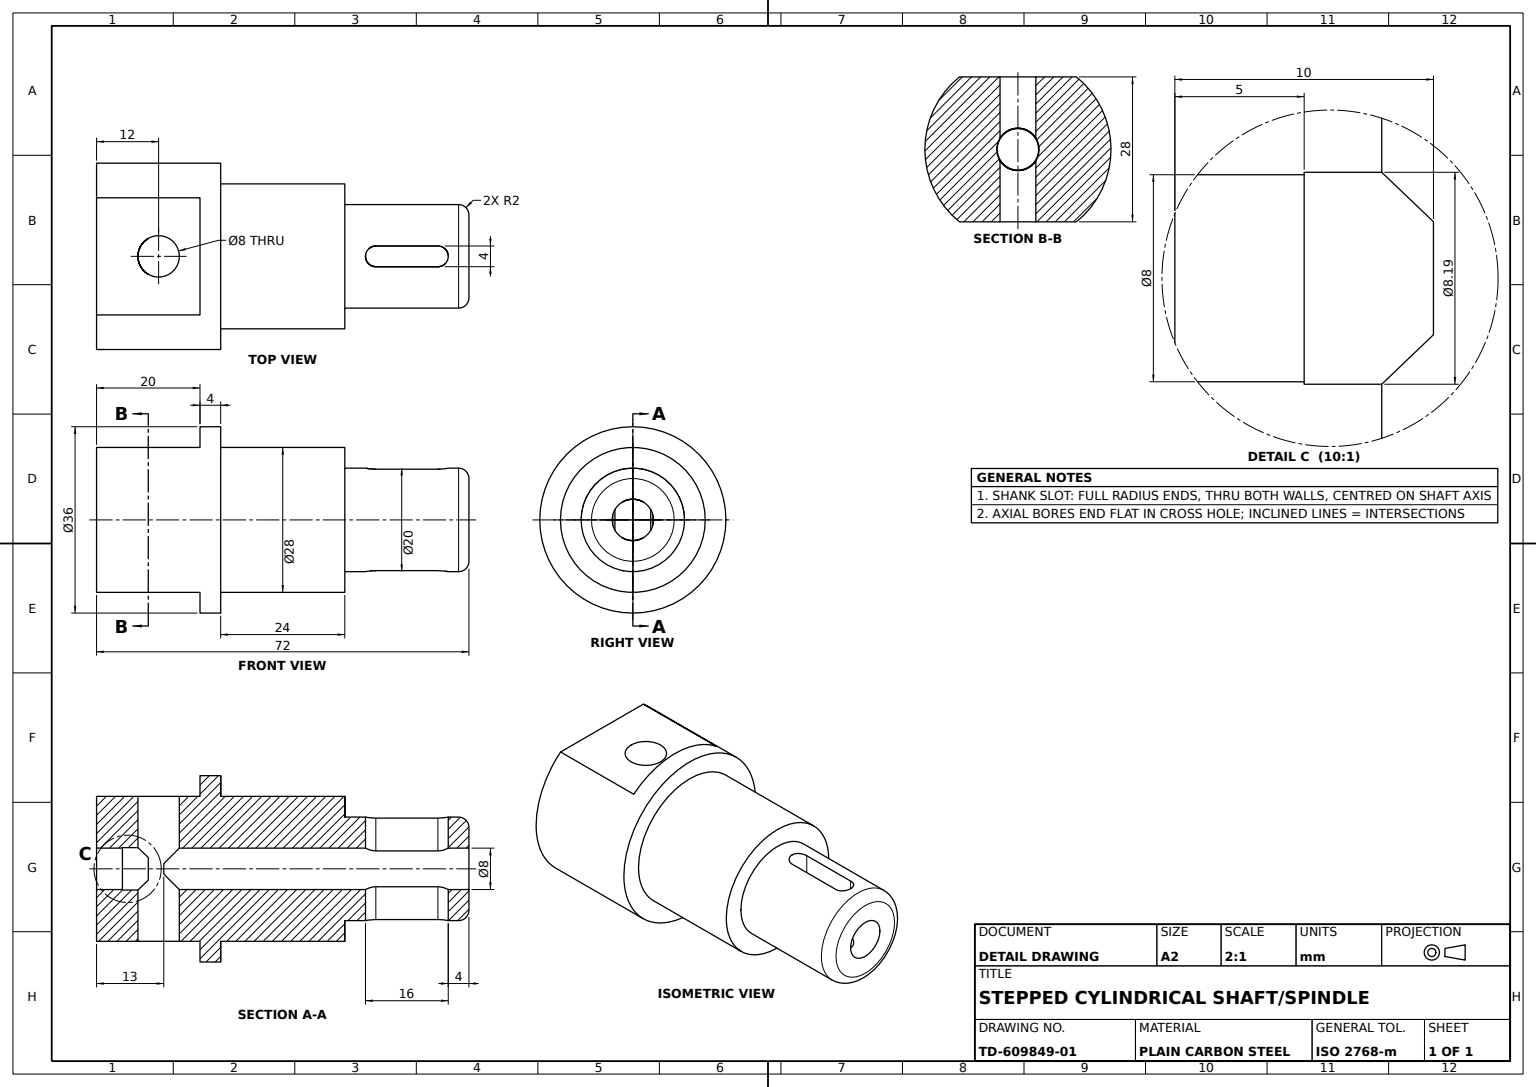
SolidWorks part; units mm, degrees
material "Plain Carbon Steel"
ref_plane "Front Plane" through (0, 0, 0) normal (0, 0, 1) x (1, 0, 0)
ref_plane "Top Plane" through (0, 0, 0) normal (0, 1, 0) x (1, 0, 0)
ref_plane "Right Plane" through (0, 0, 0) normal (1, 0, 0) x (0, 0, -1)
sketch "Shank Ø20 Sketch" plane through (0, 0, 0) normal (0, 1, 0) x (1, 0, 0)
  circle A0 centre (0, 0) radius 10
  dimension "D1" = 20
extrude "Shank Ø20 Step 1" add sketch "Shank Ø20 Sketch" along normal blind 8
sketch "Shank Step 2 Sketch" plane through (0, 8, 0) normal (0, 1, 0) x (1, 0, 0)
  circle A0 centre (0, 0) radius 10
  dimension "D1" = 20
extrude "Shank Ø20 Step 2" add sketch "Shank Step 2 Sketch" along normal blind 8
sketch "Shank Step 3 Sketch" plane through (0, 16, 0) normal (0, 1, 0) x (1, 0, 0)
  circle A0 centre (0, 0) radius 10
  dimension "D1" = 20
extrude "Shank Ø20 Step 3" add sketch "Shank Step 3 Sketch" along normal blind 8
fillet "Shank End Fillet R2" radius 2 1 edges at (0, 24, 10)
sketch "Shank Bore Ø8 Sketch" plane through (0, 24, 0) normal (0, 1, 0) x (1, 0, 0)
  circle A0 centre (0, 0) radius 4
  dimension "D1" = 8
extrude "Shank Bore Ø8 Cut 1" cut sketch "Shank Bore Ø8 Sketch" against normal blind 8
sketch "Shank Bore Cut 2 Sketch" plane through (0, 16, 0) normal (0, 1, 0) x (1, 0, 0)
  circle A0 centre (0, 0) radius 4
  dimension "D1" = 8
extrude "Shank Bore Ø8 Cut 2" cut sketch "Shank Bore Cut 2 Sketch" against normal blind 8
sketch "Shank Bore Cut 3 Sketch" plane through (0, 8, 0) normal (0, 1, 0) x (1, 0, 0)
  circle A0 centre (0, 0) radius 4
  dimension "D1" = 8
extrude "Shank Bore Ø8 Cut 3" cut sketch "Shank Bore Cut 3 Sketch" against normal blind 18
sketch "Collar Ø28 Sketch" plane through (0, 0, 0) normal (0, -1, 0) x (1, 0, 0)
  circle A0 centre (0, 0) radius 14
  dimension "D1" = 28
extrude "Collar Ø28 Step 1" add sketch "Collar Ø28 Sketch" along normal blind 8
sketch "Collar Step 2 Sketch" plane through (0, -8, 0) normal (0, -1, 0) x (1, 0, 0)
  circle A0 centre (0, 0) radius 14
  dimension "D1" = 28
extrude "Collar Ø28 Step 2" add sketch "Collar Step 2 Sketch" along normal blind 8
sketch "Collar Step 3 Sketch" plane through (0, -16, 0) normal (0, -1, 0) x (1, 0, 0)
  circle A0 centre (0, 0) radius 14
  dimension "D1" = 28
extrude "Collar Ø28 Step 3" add sketch "Collar Step 3 Sketch" along normal blind 8
sketch "Head Ø36 Sketch" plane through (0, -24, 0) normal (0, -1, 0) x (1, 0, 0)
  circle A0 centre (0, 0) radius 18
  dimension "D1" = 36
extrude "Head Ø36 Step 1" add sketch "Head Ø36 Sketch" along normal blind 8
sketch "Head Step 2 Sketch" plane through (0, -32, 0) normal (0, -1, 0) x (1, 0, 0)
  circle A0 centre (0, 0) radius 18
  dimension "D1" = 36
extrude "Head Ø36 Step 2" add sketch "Head Step 2 Sketch" along normal blind 8
sketch "Head Step 3 Sketch" plane through (0, -40, 0) normal (0, -1, 0) x (1, 0, 0)
  circle A0 centre (0, 0) radius 18
  dimension "D1" = 36
extrude "Head Ø36 Step 3" add sketch "Head Step 3 Sketch" along normal blind 8
sketch "Head Flat Sketch" plane through (0, 0, 0) normal (0, 0, 1) x (1, 0, 0)
  line L0 (-14, -48) -> (-14, -28)
  line L1 (-18, -48) -> (18, -48) construction
  line L3 (14, -28) -> (14, -48)
  line L4 (-14, -28) -> (-18, -28)
  line L5 (-14, -28) -> (14, -28)
  line L6 (-18, -28) -> (18, -28)
  line L7 (-18, -48) -> (-18, -28)
  line L8 (18, -48) -> (18, -28)
  line L9 (-18, -48) -> (18, -48)
  dimension "D1" = 4
  dimension "D2" = 32
  dimension "D3" = 20
extrude "Head Flat" cut sketch "Head Flat Sketch" against normal blind 40 and the other way blind 51 contours L7 L9 L0 L4 | L3 L9 L8 L6
sketch "Cross Hole Ø8 Sketch" plane through (14, 0, 0) normal (1, 0, 0) x (0, 0, -1)
  circle A0 centre (0, -36) radius 4
  dimension "D1" = 8
  dimension "D2" = 12
  dimension "D3" = 11.3137
extrude "Cross Hole Ø8" cut sketch "Cross Hole Ø8 Sketch" against normal blind 52 and the other way blind 20
sketch "Collar Bore Cut 1 Sketch" plane through (0, 0, 0) normal (0, 1, 0) x (1, 0, 0)
  circle A0 centre (0, 0) radius 4
  dimension "D1" = 8
extrude "Collar Bore Cut 1" cut sketch "Collar Bore Cut 1 Sketch" against normal blind 5
sketch "Collar Bore Cut 2 Sketch" plane through (0, -5, 0) normal (0, 1, 0) x (1, 0, 0)
  circle A0 centre (0, 0) radius 4
  dimension "D1" = 8
extrude "Collar Bore Cut 2" cut sketch "Collar Bore Cut 2 Sketch" against normal blind 5
sketch "Collar Bore Cut 3 Sketch" plane through (0, -10, 0) normal (0, 1, 0) x (1, 0, 0)
  circle A0 centre (0, 0) radius 4
  dimension "D1" = 8
extrude "Collar Bore Cut 3" cut sketch "Collar Bore Cut 3 Sketch" against normal blind 5
sketch "Head Bore Ø8 Sketch" plane through (0, -48, 0) normal (0, -1, 0) x (1, 0, 0)
  circle A0 centre (0, 0) radius 4
  dimension "D1" = 8
extrude "Head Bore Ø8 Cut 1" cut sketch "Head Bore Ø8 Sketch" against normal blind 5
sketch "Head Bore Cut 2 Sketch" plane through (0, -43, 0) normal (0, -1, 0) x (1, 0, 0)
  circle A0 centre (0, 0) radius 4.0947
  dimension "D1" = 8.1893
extrude "Head Bore Ø8 Cut 2" cut sketch "Head Bore Cut 2 Sketch" against normal blind 5
sketch "Collar Bore Cut 4 Sketch" plane through (0, -15, 0) normal (0, 1, 0) x (1, 0, 0)
  circle A0 centre (0, 0) radius 4
  dimension "D1" = 8
extrude "Collar Bore Cut 4" cut sketch "Collar Bore Cut 4 Sketch" against normal blind 5
sketch "Inner Bore Ø8 Sketch" plane through (0, -20, 0) normal (0, 1, 0) x (1, 0, 0)
  circle A0 centre (0, 0) radius 4
  dimension "D1" = 8
extrude "Inner Bore Ø8 Cut 1" cut sketch "Inner Bore Ø8 Sketch" against normal blind 5
sketch "Inner Bore Cut 2 Sketch" plane through (0, -25, 0) normal (0, 1, 0) x (1, 0, 0)
  circle A0 centre (0, 0) radius 4
  dimension "D1" = 8
extrude "Inner Bore Ø8 Cut 2" cut sketch "Inner Bore Cut 2 Sketch" against normal blind 5
sketch "Inner Bore Cut 3 Sketch" plane through (0, -30, 0) normal (0, 1, 0) x (1, 0, 0)
  circle A0 centre (0, 0) radius 4
  dimension "D1" = 8
extrude "Inner Bore Ø8 Cut 3" cut sketch "Inner Bore Cut 3 Sketch" against normal blind 5
sketch "Shank Slot Sketch" plane through (14, 0, 0) normal (1, 0, 0) x (0, 0, -1)
  line L1 (-2, 18) -> (-2, 6)
  line L2 (2, 18) -> (2, 6)
  arc A0 (2, 18) -> (-2, 18) centre (0, 18) ccw
  arc A1 (-2, 6) -> (2, 6) centre (0, 6) ccw
  dimension "D3" = 4
  dimension "D4" = 4
  dimension "D1" = 12
  dimension "D2" = 6
extrude "Shank Slot" cut sketch "Shank Slot Sketch" against normal blind 146 and the other way blind 137
